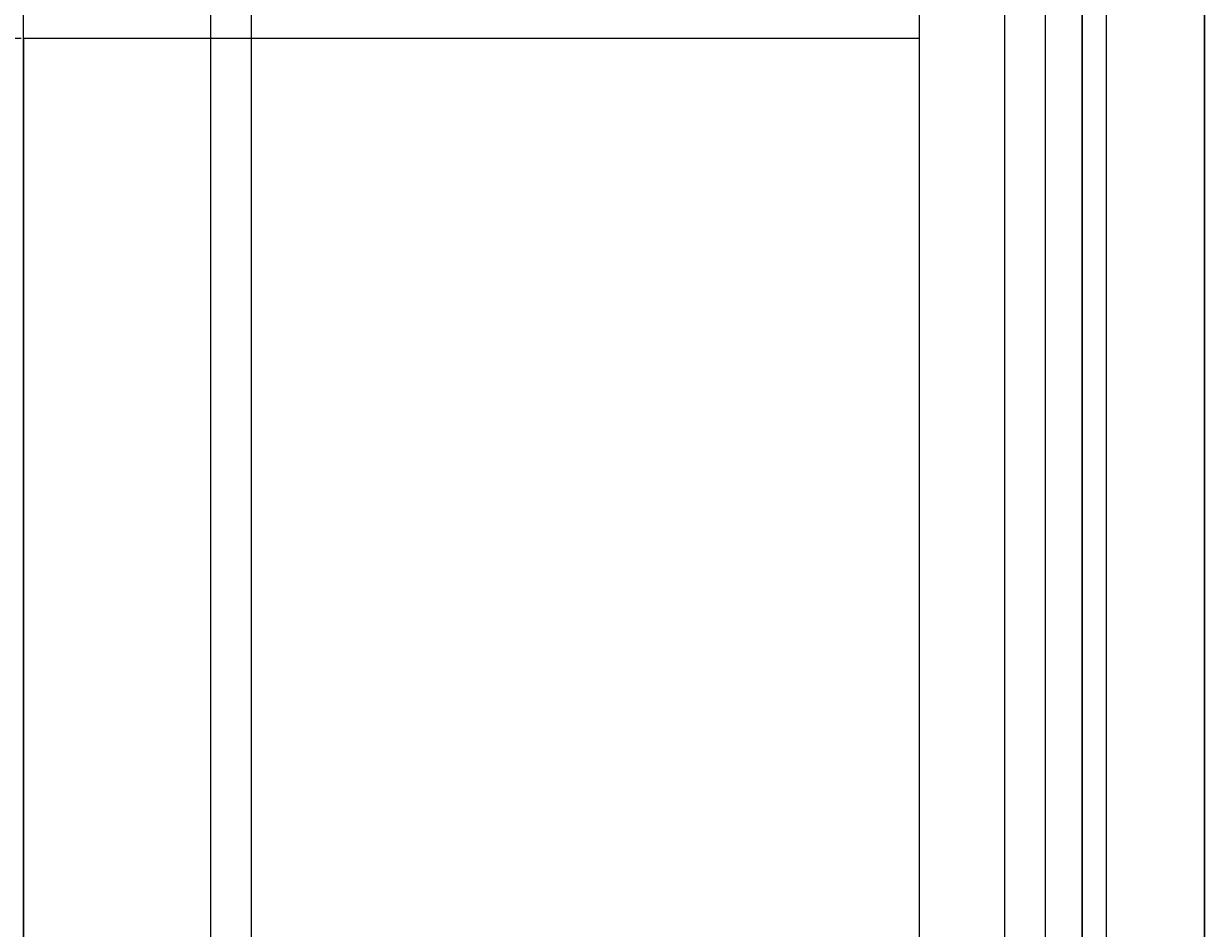
# Model space of a CAD drawing. Units: inches. Extents: x -6 to 289, y -8 to 323.
# Tile 26 of 107: x 142 to 171, y 87 to 109. Entities that reach past the tile are written whole.
import ezdxf

# ---------------------------------------------------------------- set-up
doc = ezdxf.new("R2010")
doc.units = ezdxf.units.IN
doc.header["$MEASUREMENT"] = 0
doc.layers.add('A-ANNO-DIMS', color=2, linetype='Continuous', lineweight=18)
doc.layers.add('A-DOOR', color=3, linetype='Continuous', lineweight=25)
doc.styles.get("Standard").update_dxf_attribs({"font": 'arial.ttf'})
doc.dimstyles.get("Standard").update_dxf_attribs({"dimtxt": 0.18, "dimasz": 0.18, "dimexe": 0.18, "dimexo": 0.0625, "dimgap": 0.09, "dimtad": 0, "dimtih": 1, "dimtoh": 1, "dimdec": 4, "dimzin": 0, "dimdsep": 46, "dimtxsty": 'Standard', "dimcen": 0.09, "dimadec": 0, "dimazin": 0, "dimtfac": 1, "dimtdec": 4, "dimtofl": 0, "dimtmove": 0, "dimatfit": 3, "dimfxl": 1, "dimtolj": 1, "dimtzin": 0, "dimarcsym": 0})

# ---------------------------------------------------------------- blocks, each defined once
blk = doc.blocks.new('*D30')
at = {"layer": 'A-ANNO-DIMS', "color": 0, "lineweight": -2, "transparency": 16777216}
for p, q in [((129.383, 181.092), (129.383, -8.391)), ((146.883, 181.092), (146.883, -8.391)), ((129.563, -8.211), (137.817, -8.211)), ((146.703, -8.211), (138.449, -8.211))]:
    blk.add_line(p, q, dxfattribs=at)
at = {"layer": 'A-ANNO-DIMS', "color": 0, "transparency": 16777216}
for points in [[(129.563, -8.181), (129.563, -8.241), (129.383, -8.211)], [(146.703, -8.181), (146.703, -8.241), (146.883, -8.211)]]:
    blk.add_solid(points, dxfattribs=at)
at = {"layer": 'Defpoints', "color": 0, "transparency": 16777216}
for p in [(129.383, 181.154), (146.883, 181.154), (146.883, -8.211)]:
    blk.add_point(p, dxfattribs=at)
at = {"layer": 'A-ANNO-DIMS', "color": 0, "transparency": 16777216, "insert": (138.133, -8.211), "char_height": 0.18, "attachment_point": 5}
blk.add_mtext('\\A1;17.5', dxfattribs=at)
blk = doc.blocks.new('*D31')
at = {"layer": 'A-ANNO-DIMS', "color": 0, "lineweight": -2, "transparency": 16777216}
for p, q in [((146.883, 181.092), (146.883, -8.391)), ((147.883, 181.092), (147.883, -8.391)), ((147.063, -8.211), (147.26, -8.211)), ((147.703, -8.211), (147.507, -8.211))]:
    blk.add_line(p, q, dxfattribs=at)
at = {"layer": 'A-ANNO-DIMS', "color": 0, "transparency": 16777216}
for points in [[(147.063, -8.181), (147.063, -8.241), (146.883, -8.211)], [(147.703, -8.181), (147.703, -8.241), (147.883, -8.211)]]:
    blk.add_solid(points, dxfattribs=at)
at = {"layer": 'Defpoints', "color": 0, "transparency": 16777216}
for p in [(146.883, 181.154), (147.883, 181.154), (147.883, -8.211)]:
    blk.add_point(p, dxfattribs=at)
at = {"layer": 'A-ANNO-DIMS', "color": 0, "transparency": 16777216, "insert": (147.383, -8.211), "char_height": 0.18, "attachment_point": 5}
blk.add_mtext('\\A1;1', dxfattribs=at)
blk = doc.blocks.new('*D32')
at = {"layer": 'A-ANNO-DIMS', "color": 0, "lineweight": -2, "transparency": 16777216}
for p, q in [((147.883, 181.092), (147.883, -8.391)), ((166.383, 181.092), (166.383, -8.391)), ((148.063, -8.211), (156.817, -8.211)), ((166.203, -8.211), (157.449, -8.211))]:
    blk.add_line(p, q, dxfattribs=at)
at = {"layer": 'A-ANNO-DIMS', "color": 0, "transparency": 16777216}
for points in [[(148.063, -8.181), (148.063, -8.241), (147.883, -8.211)], [(166.203, -8.181), (166.203, -8.241), (166.383, -8.211)]]:
    blk.add_solid(points, dxfattribs=at)
at = {"layer": 'Defpoints', "color": 0, "transparency": 16777216}
for p in [(147.883, 181.154), (166.383, 181.154), (166.383, -8.211)]:
    blk.add_point(p, dxfattribs=at)
at = {"layer": 'A-ANNO-DIMS', "color": 0, "transparency": 16777216, "insert": (157.133, -8.211), "char_height": 0.18, "attachment_point": 5}
blk.add_mtext('\\A1;18.5', dxfattribs=at)
blk = doc.blocks.new('*D33')
at = {"layer": 'A-ANNO-DIMS', "color": 0, "lineweight": -2, "transparency": 16777216}
for p, q in [((166.383, 181.092), (166.383, -8.391)), ((167.383, 180.092), (167.383, -8.391)), ((166.563, -8.211), (166.76, -8.211)), ((167.203, -8.211), (167.007, -8.211))]:
    blk.add_line(p, q, dxfattribs=at)
at = {"layer": 'A-ANNO-DIMS', "color": 0, "transparency": 16777216}
for points in [[(166.563, -8.181), (166.563, -8.241), (166.383, -8.211)], [(167.203, -8.181), (167.203, -8.241), (167.383, -8.211)]]:
    blk.add_solid(points, dxfattribs=at)
at = {"layer": 'Defpoints', "color": 0, "transparency": 16777216}
for p in [(166.383, 181.154), (167.383, 180.154), (167.383, -8.211)]:
    blk.add_point(p, dxfattribs=at)
at = {"layer": 'A-ANNO-DIMS', "color": 0, "transparency": 16777216, "insert": (166.883, -8.211), "char_height": 0.18, "attachment_point": 5}
blk.add_mtext('\\A1;1', dxfattribs=at)
blk = doc.blocks.new('*D34')
at = {"layer": 'A-ANNO-DIMS', "color": 0, "lineweight": -2, "transparency": 16777216}
for p, q in [((167.383, 180.092), (167.383, -8.391)), ((168.883, 178.592), (168.883, -8.391)), ((167.563, -8.211), (167.887, -8.211)), ((168.703, -8.211), (168.38, -8.211))]:
    blk.add_line(p, q, dxfattribs=at)
at = {"layer": 'A-ANNO-DIMS', "color": 0, "transparency": 16777216}
for points in [[(167.563, -8.181), (167.563, -8.241), (167.383, -8.211)], [(168.703, -8.181), (168.703, -8.241), (168.883, -8.211)]]:
    blk.add_solid(points, dxfattribs=at)
at = {"layer": 'Defpoints', "color": 0, "transparency": 16777216}
for p in [(167.383, 180.154), (168.883, 178.654), (168.883, -8.211)]:
    blk.add_point(p, dxfattribs=at)
at = {"layer": 'A-ANNO-DIMS', "color": 0, "transparency": 16777216, "insert": (168.133, -8.211), "char_height": 0.18, "attachment_point": 5}
blk.add_mtext('\\A1;1.5', dxfattribs=at)
blk = doc.blocks.new('*D76')
at = {"layer": 'A-ANNO-DIMS', "color": 0, "lineweight": -2, "transparency": 16777216}
for p, q in [((142.296, 51.148), (142.296, 322.969)), ((142.476, 322.789), (153.076, 322.789)), ((164.116, 322.789), (153.516, 322.789)), ((164.296, 51.148), (164.296, 322.969))]:
    blk.add_line(p, q, dxfattribs=at)
at = {"layer": 'A-ANNO-DIMS', "color": 0, "transparency": 16777216}
for points in [[(142.476, 322.819), (142.476, 322.759), (142.296, 322.789)], [(164.116, 322.819), (164.116, 322.759), (164.296, 322.789)]]:
    blk.add_solid(points, dxfattribs=at)
at = {"layer": 'Defpoints', "color": 0, "transparency": 16777216}
for p in [(164.296, 322.789), (142.296, 51.085), (164.296, 51.085)]:
    blk.add_point(p, dxfattribs=at)
at = {"layer": 'A-ANNO-DIMS', "color": 0, "transparency": 16777216, "insert": (153.296, 322.789), "char_height": 0.18, "attachment_point": 5}
blk.add_mtext('\\A1;22', dxfattribs=at)
blk = doc.blocks.new('*D77')
at = {"layer": 'A-ANNO-DIMS', "color": 0, "lineweight": -2, "transparency": 16777216}
for p, q in [((164.296, 51.148), (164.296, 322.969)), ((164.476, 322.789), (166.144, 322.789)), ((168.116, 322.789), (166.448, 322.789)), ((168.296, 51.148), (168.296, 322.969))]:
    blk.add_line(p, q, dxfattribs=at)
at = {"layer": 'A-ANNO-DIMS', "color": 0, "transparency": 16777216}
for points in [[(164.476, 322.819), (164.476, 322.759), (164.296, 322.789)], [(168.116, 322.819), (168.116, 322.759), (168.296, 322.789)]]:
    blk.add_solid(points, dxfattribs=at)
at = {"layer": 'Defpoints', "color": 0, "transparency": 16777216}
for p in [(168.296, 322.789), (164.296, 51.085), (168.296, 51.085)]:
    blk.add_point(p, dxfattribs=at)
at = {"layer": 'A-ANNO-DIMS', "color": 0, "transparency": 16777216, "insert": (166.296, 322.789), "char_height": 0.18, "attachment_point": 5}
blk.add_mtext('\\A1;4', dxfattribs=at)
blk = doc.blocks.new('*D78')
at = {"layer": 'A-ANNO-DIMS', "color": 0, "lineweight": -2, "transparency": 16777216}
for p, q in [((168.296, 51.148), (168.296, 322.969)), ((168.476, 322.789), (169.647, 322.789)), ((171.116, 322.789), (169.945, 322.789)), ((171.296, 51.148), (171.296, 322.969))]:
    blk.add_line(p, q, dxfattribs=at)
at = {"layer": 'A-ANNO-DIMS', "color": 0, "transparency": 16777216}
for points in [[(168.476, 322.819), (168.476, 322.759), (168.296, 322.789)], [(171.116, 322.819), (171.116, 322.759), (171.296, 322.789)]]:
    blk.add_solid(points, dxfattribs=at)
at = {"layer": 'Defpoints', "color": 0, "transparency": 16777216}
for p in [(171.296, 322.789), (168.296, 51.085), (171.296, 51.085)]:
    blk.add_point(p, dxfattribs=at)
at = {"layer": 'A-ANNO-DIMS', "color": 0, "transparency": 16777216, "insert": (169.796, 322.789), "char_height": 0.18, "attachment_point": 5}
blk.add_mtext('\\A1;3', dxfattribs=at)
blk = doc.blocks.new('*D87')
at = {"layer": 'A-ANNO-DIMS', "color": 0, "lineweight": -2, "transparency": 16777216}
for p, q in [((142.233, 108.948), (-5.737, 108.948)), ((-5.557, 108.768), (-5.557, 92.641)), ((-5.557, 76.151), (-5.557, 92.277)), ((166.233, 75.971), (-5.737, 75.971))]:
    blk.add_line(p, q, dxfattribs=at)
at = {"layer": 'A-ANNO-DIMS', "color": 0, "transparency": 16777216}
for points in [[(-5.587, 108.768), (-5.527, 108.768), (-5.557, 108.948)], [(-5.587, 76.151), (-5.527, 76.151), (-5.557, 75.971)]]:
    blk.add_solid(points, dxfattribs=at)
at = {"layer": 'Defpoints', "color": 0, "transparency": 16777216}
for p in [(-5.557, 108.948), (142.296, 108.948), (166.296, 75.971)]:
    blk.add_point(p, dxfattribs=at)
at = {"layer": 'A-ANNO-DIMS', "color": 0, "transparency": 16777216, "insert": (-5.557, 92.459), "char_height": 0.18, "attachment_point": 5}
blk.add_mtext('\\A1;32.98', dxfattribs=at)

msp = doc.modelspace()

# ---------------------------------------------------------------- linework, layer by layer
at = {"layer": 'A-DOOR'}
for points in [[(135.296, 51.0851), (135.296, 117.9706), (171.296, 117.9706), (171.296, 51.0851)], [(138.296, 51.0851), (138.296, 114.9477), (168.296, 114.9477), (168.296, 51.0851)], [(164.296, 51.0851), (164.296, 108.9477), (142.296, 108.9477), (142.296, 51.0851)]]:
    msp.add_lwpolyline(points, dxfattribs=at)

# ---------------------------------------------------------------- dimensions: what is measured, and where the dimension line sits
at = {"layer": 'A-ANNO-DIMS'}
for base, p1, p2, override, picture, middle in [((164.296, 322.7888), (142.296, 51.0851), (164.296, 51.0851), {"dimdec": 0, "dimlfac": 1, "dimrnd": 0, "dimzin": 0, "dimdsep": 46, "dimlunit": 2}, '*D76', (153.296, 322.7888)), ((168.296, 322.7888), (164.296, 51.0851), (168.296, 51.0851), {"dimdec": 0, "dimlfac": 1, "dimrnd": 0, "dimzin": 0, "dimdsep": 46, "dimlunit": 2}, '*D77', (166.296, 322.7888)), ((171.296, 322.7888), (168.296, 51.0851), (171.296, 51.0851), {"dimdec": 0, "dimlfac": 1, "dimrnd": 0, "dimzin": 0, "dimdsep": 46, "dimlunit": 2}, '*D78', (169.796, 322.7888)), ((146.8835, -8.2112), (129.3835, 181.154), (146.8835, 181.154), {"dimdec": 1, "dimlfac": 1, "dimrnd": 0, "dimzin": 0, "dimdsep": 46, "dimlunit": 2}, '*D30', (138.1335, -8.2112)), ((147.8835, -8.2112), (146.8835, 181.154), (147.8835, 181.154), {"dimdec": 0, "dimlfac": 1, "dimrnd": 0, "dimzin": 0, "dimdsep": 46, "dimlunit": 2}, '*D31', (147.3835, -8.2112)), ((166.3835, -8.2112), (147.8835, 181.154), (166.3835, 181.154), {"dimdec": 1, "dimlfac": 1, "dimrnd": 0, "dimzin": 0, "dimdsep": 46, "dimlunit": 2}, '*D32', (157.1335, -8.2112)), ((167.3835, -8.2112), (166.3835, 181.154), (167.3835, 180.154), {"dimdec": 0, "dimlfac": 1, "dimrnd": 0, "dimzin": 0, "dimdsep": 46, "dimlunit": 2}, '*D33', (166.8835, -8.2112)), ((168.8835, -8.2112), (167.3835, 180.154), (168.8835, 178.654), {"dimdec": 1, "dimlfac": 1, "dimrnd": 0, "dimzin": 0, "dimdsep": 46, "dimlunit": 2}, '*D34', (168.1335, -8.2112))]:
    dim = msp.add_linear_dim(base=base, p1=p1, p2=p2, dimstyle='Standard', override=override, dxfattribs=at)
    dim.commit()
    dim.dimension.update_dxf_attribs({"geometry": picture, "text_midpoint": middle})
dim = msp.add_linear_dim(base=(-5.557, 108.9477), p1=(166.296, 75.9706), p2=(142.296, 108.9477), angle=90, dimstyle='Standard', override={"dimdec": 2, "dimlfac": 1, "dimrnd": 0, "dimzin": 0, "dimdsep": 46, "dimlunit": 2}, dxfattribs=at)
dim.commit()
dim.dimension.update_dxf_attribs({"geometry": '*D87', "text_midpoint": (-5.557, 92.4592)})

doc.saveas('drawing.dxf')
